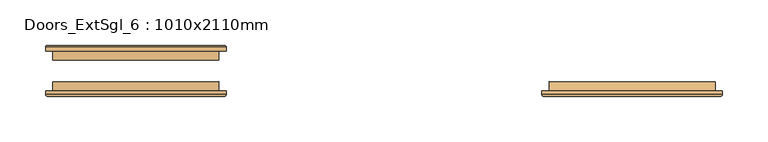
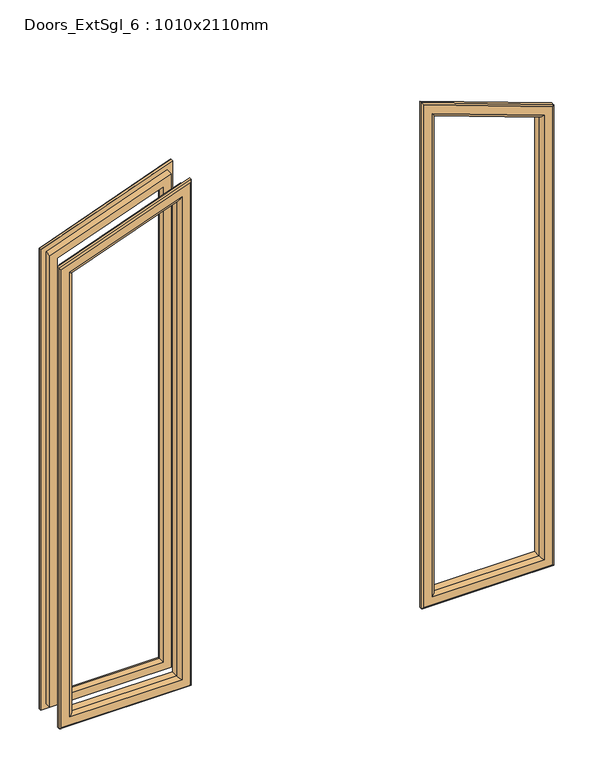
"""IFC4 building model written with IfcOpenShell, lengths in millimetres: door geometry, Doors_ExtSgl_6 : 1010x2110mm."""

from ifc_helpers import new_model, si_unit, frame, origin, place, context, project, spatial, ellipse_curve, source, transform, mapped, element, save
from ifc_brep_helpers import plane_surface, cylinder_surface, advanced_brep


def doors_extsgl_6_1010x2110mm_efbaf1af(model_context):
    return source(origin(), model_context, "Body", "AdvancedBrep", [
        advanced_brep(
        [(363.5333333, -2.4, 1776.1968198), (363.5333333, -12.4, 1776.1968198), (363.5333333, -12.4, 1058.5), (363.5333333, -2.4, 1058.5), (351.5333333, -13.4, 1767.7943294), (351.5333333, -2.4, 1767.7943294), (351.5333333, -2.4, 1070.5), (351.5333333, -13.4, 1070.5), (356.5333333, -18.4, 1771.2953671), (356.5333333, -18.4, 1065.5), (371.5333333, -16.4, 1781.7984801), (369.5333333, -18.4, 1780.3980651), (369.5333333, -18.4, 1052.5), (371.5333333, -16.4, 1050.5), (371.5333333, -12.4, 1781.7984801), (371.5333333, -12.4, 1050.5), (181.2, -12.4, 1058.5), (181.2, -2.4, 1058.5), (193.2, -2.4, 1070.5), (193.2, -13.4, 1070.5), (188.2, -18.4, 1065.5), (175.2, -18.4, 1052.5), (173.2, -16.4, 1050.5), (173.2, -12.4, 1050.5), (181.2, -12.4, 1842.5607259), (181.2, -2.4, 1842.5607259), (193.2, -2.4, 1825.4229498), (193.2, -13.4, 1825.4229498), (188.2, -18.4, 1832.5636898), (175.2, -18.4, 1851.1296139), (173.2, -16.4, 1853.9859099), (173.2, -12.4, 1853.9859099)],
        [
            (0, 1),
            (1, 2),
            (2, 3),
            (3, 0),
            (4, 5),
            (5, 6),
            (6, 7),
            (7, 4),
            (8, 4, ellipse_curve(frame((356.5333333, -13.4, 1771.2953671), z_axis=(0.5735764363510455, 0.0, -0.8191520442889922), x_axis=(0.8191520442889922, 0.0, 0.5735764363510455)), 6.1038729, 5.0)),
            (7, 9, ellipse_curve(frame((356.5333333, -13.4, 1065.5), z_axis=(0.7071067811865475, 0.0, 0.7071067811865475), x_axis=(-0.7071067811865474, 0.0, 0.7071067811865476)), 7.0710678, 5.0)),
            (9, 8),
            (10, 11, ellipse_curve(frame((369.5333333, -16.4, 1780.3980651), z_axis=(0.5735764363510455, 0.0, -0.8191520442889922), x_axis=(0.8191520442889922, 0.0, 0.5735764363510455)), 2.4415492, 2.0)),
            (11, 12),
            (12, 13, ellipse_curve(frame((369.5333333, -16.4, 1052.5), z_axis=(0.7071067811865475, 0.0, 0.7071067811865475), x_axis=(-0.7071067811865474, 0.0, 0.7071067811865476)), 2.8284271, 2.0)),
            (13, 10),
            (14, 10),
            (13, 15),
            (15, 14),
            (2, 16),
            (16, 17),
            (17, 3),
            (6, 18),
            (18, 19),
            (19, 7),
            (19, 20, ellipse_curve(frame((188.2, -13.4, 1065.5), z_axis=(0.7071067811865475, 0.0, -0.7071067811865475), x_axis=(0.7071067811865476, 0.0, 0.7071067811865474)), 7.0710678, 5.0)),
            (20, 9),
            (12, 21),
            (21, 22, ellipse_curve(frame((175.2, -16.4, 1052.5), z_axis=(0.7071067811865475, 0.0, -0.7071067811865475), x_axis=(0.7071067811865476, 0.0, 0.7071067811865474)), 2.8284271, 2.0)),
            (22, 13),
            (22, 23),
            (23, 15),
            (16, 24),
            (24, 25),
            (25, 17),
            (18, 26),
            (26, 27),
            (27, 19),
            (27, 28, ellipse_curve(frame((188.2, -13.4, 1832.5636898), z_axis=(-0.8191520442889922, 0.0, -0.5735764363510455), x_axis=(0.5735764363510455, 0.0, -0.8191520442889922)), 8.717234, 5.0)),
            (28, 20),
            (21, 29),
            (29, 30, ellipse_curve(frame((175.2, -16.4, 1851.1296139), z_axis=(-0.8191520442889922, 0.0, -0.5735764363510455), x_axis=(0.5735764363510455, 0.0, -0.8191520442889922)), 3.4868936, 2.0)),
            (30, 22),
            (30, 31),
            (31, 23),
            (31, 14),
            (1, 24),
            (0, 25),
            (5, 26),
            (4, 27),
            (8, 28),
            (11, 29),
            (10, 30),
        ],
        [
            plane_surface(frame((363.5333333, -12.4, 1776.1968198), z_axis=(1.0, 0.0, 0.0), x_axis=(0.0, 0.0, -1.0))),
            plane_surface(frame((351.5333333, -2.4, 1767.7943294), z_axis=(-1.0, 0.0, 0.0), x_axis=(0.0, 0.0, -1.0))),
            cylinder_surface(frame((356.5333333, -13.4, 1776.1968198), z_axis=(0.0, 0.0, 1.0), x_axis=(1.0, 0.0, 0.0)), 5.0),
            cylinder_surface(frame((369.5333333, -16.4, 1776.1968198), z_axis=(0.0, 0.0, 1.0), x_axis=(1.0, 0.0, 0.0)), 2.0),
            plane_surface(frame((371.5333333, -16.4, 1781.7984801), z_axis=(1.0, 0.0, 0.0), x_axis=(0.0, 0.0, -1.0))),
            plane_surface(frame((363.5333333, -12.4, 1058.5), z_axis=(0.0, 0.0, -1.0), x_axis=(-1.0, 0.0, 0.0))),
            plane_surface(frame((351.5333333, -2.4, 1070.5), z_axis=(0.0, 0.0, 1.0), x_axis=(-1.0, 0.0, 0.0))),
            cylinder_surface(frame((363.5333333, -13.4, 1065.5), z_axis=(1.0, 0.0, 0.0), x_axis=(0.0, 0.0, -1.0)), 5.0),
            cylinder_surface(frame((363.5333333, -16.4, 1052.5), z_axis=(1.0, 0.0, 0.0), x_axis=(0.0, 0.0, -1.0)), 2.0),
            plane_surface(frame((371.5333333, -16.4, 1050.5), z_axis=(0.0, 0.0, -1.0), x_axis=(-1.0, 0.0, 0.0))),
            plane_surface(frame((181.2, -12.4, 1058.5), z_axis=(-1.0, 0.0, 0.0), x_axis=(0.0, 0.0, 1.0))),
            plane_surface(frame((193.2, -2.4, 1070.5), z_axis=(1.0, 0.0, 0.0), x_axis=(0.0, 0.0, 1.0))),
            cylinder_surface(frame((188.2, -13.4, 1058.5), z_axis=(0.0, 0.0, -1.0), x_axis=(-1.0, 0.0, 0.0)), 5.0),
            cylinder_surface(frame((175.2, -16.4, 1058.5), z_axis=(0.0, 0.0, -1.0), x_axis=(-1.0, 0.0, 0.0)), 2.0),
            plane_surface(frame((173.2, -16.4, 1050.5), z_axis=(-1.0, 0.0, 0.0), x_axis=(0.0, 0.0, 1.0))),
            plane_surface(frame((173.2, -12.4, 1853.9859099), z_axis=(0.0, 1.0000000000000002, 0.0), x_axis=(0.9396926207859078, 0.0, -0.3420201433256707))),
            plane_surface(frame((181.2, -12.4, 1842.5607259), z_axis=(0.3420201433256708, 0.0, 0.9396926207859077), x_axis=(0.9396926207859077, 0.0, -0.3420201433256708))),
            plane_surface(frame((181.2, -2.4, 1842.5607259), z_axis=(0.0, 1.0000000000000002, 0.0), x_axis=(0.939692620785908, 0.0, -0.34202014332567))),
            plane_surface(frame((193.2, -2.4, 1825.4229498), z_axis=(-0.34202014332566955, 0.0, -0.9396926207859082), x_axis=(0.9396926207859082, 0.0, -0.34202014332566955))),
            cylinder_surface(frame((178.805859, -13.4, 1835.9828775), z_axis=(-0.9396926207859079, 0.0, 0.34202014332567016), x_axis=(0.34202014332567016, 0.0, 0.9396926207859079)), 5.0),
            plane_surface(frame((188.2, -18.4, 1832.5636898), z_axis=(0.0, -1.0, 0.0), x_axis=(0.9396926207859079, 0.0, -0.34202014332567027))),
            cylinder_surface(frame((183.2521209, -16.4, 1848.1988816), z_axis=(-0.9396926207859079, 0.0, 0.34202014332567016), x_axis=(0.34202014332567016, 0.0, 0.9396926207859079)), 2.0),
            plane_surface(frame((173.2, -16.4, 1853.9859099), z_axis=(0.3420201433256701, 0.0, 0.939692620785908), x_axis=(0.939692620785908, 0.0, -0.3420201433256701))),
        ],
        [
            (0, [[1, 2, 3, 4]]),
            (1, [[5, 6, 7, 8]]),
            (2, [[9, -8, 10, 11]]),
            (3, [[12, 13, 14, 15]]),
            (4, [[16, -15, 17, 18]]),
            (5, [[-3, 19, 20, 21]]),
            (6, [[-7, 22, 23, 24]]),
            (7, [[-10, -24, 25, 26]]),
            (8, [[-14, 27, 28, 29]]),
            (9, [[-17, -29, 30, 31]]),
            (10, [[-20, 32, 33, 34]]),
            (11, [[-23, 35, 36, 37]]),
            (12, [[-25, -37, 38, 39]]),
            (13, [[-28, 40, 41, 42]]),
            (14, [[-30, -42, 43, 44]]),
            (15, [[-31, -44, 45, -18], [46, -32, -19, -2]]),
            (16, [[-33, -46, -1, 47]]),
            (17, [[-21, -34, -47, -4], [48, -35, -22, -6]]),
            (18, [[-36, -48, -5, 49]]),
            (19, [[-38, -49, -9, 50]]),
            (20, [[51, -40, -27, -13], [-26, -39, -50, -11]]),
            (21, [[-41, -51, -12, 52]]),
            (22, [[-43, -52, -16, -45]]),
        ],
    ),
        advanced_brep(
        [(-173.1333333, 35.6, 1050.5), (-173.1333333, 31.6, 1050.5), (-371.4666667, 31.6, 1050.5), (-371.4666667, 35.6, 1050.5), (-175.1333333, 37.6, 1052.5), (-369.4666667, 37.6, 1052.5), (-193.1333333, 32.6, 1070.5), (-188.1333333, 37.6, 1065.5), (-356.4666667, 37.6, 1065.5), (-351.4666667, 32.6, 1070.5), (-193.1333333, 21.6, 1070.5), (-351.4666667, 21.6, 1070.5), (-181.1333333, 31.6, 1058.5), (-181.1333333, 21.6, 1058.5), (-363.4666667, 21.6, 1058.5), (-363.4666667, 31.6, 1058.5), (-371.4666667, 31.6, 1781.7984801), (-371.4666667, 35.6, 1781.7984801), (-369.4666667, 37.6, 1780.3980651), (-356.4666667, 37.6, 1771.2953671), (-351.4666667, 32.6, 1767.7943294), (-351.4666667, 21.6, 1767.7943294), (-363.4666667, 21.6, 1776.1968198), (-363.4666667, 31.6, 1776.1968198), (-173.1333333, 31.6, 1853.9859099), (-173.1333333, 35.6, 1853.9859099), (-175.1333333, 37.6, 1851.1296139), (-188.1333333, 37.6, 1832.5636898), (-193.1333333, 32.6, 1825.4229498), (-193.1333333, 21.6, 1825.4229498), (-181.1333333, 21.6, 1842.5607259), (-181.1333333, 31.6, 1842.5607259)],
        [
            (0, 1),
            (1, 2),
            (2, 3),
            (3, 0),
            (4, 0, ellipse_curve(frame((-175.1333333, 35.6, 1052.5), z_axis=(-0.7071067811865475, 0.0, -0.7071067811865475), x_axis=(0.7071067811865477, 0.0, -0.7071067811865474)), 2.8284271, 2.0)),
            (3, 5, ellipse_curve(frame((-369.4666667, 35.6, 1052.5), z_axis=(0.7071067811865475, 0.0, -0.7071067811865475), x_axis=(0.7071067811865476, 0.0, 0.7071067811865474)), 2.8284271, 2.0)),
            (5, 4),
            (6, 7, ellipse_curve(frame((-188.1333333, 32.6, 1065.5), z_axis=(-0.7071067811865475, 0.0, -0.7071067811865475), x_axis=(0.7071067811865477, 0.0, -0.7071067811865474)), 7.0710678, 5.0)),
            (7, 8),
            (8, 9, ellipse_curve(frame((-356.4666667, 32.6, 1065.5), z_axis=(0.7071067811865475, 0.0, -0.7071067811865475), x_axis=(0.7071067811865476, 0.0, 0.7071067811865474)), 7.0710678, 5.0)),
            (9, 6),
            (10, 6),
            (9, 11),
            (11, 10),
            (12, 13),
            (13, 14),
            (14, 15),
            (15, 12),
            (2, 16),
            (16, 17),
            (17, 3),
            (17, 18, ellipse_curve(frame((-369.4666667, 35.6, 1780.3980651), z_axis=(-0.5735764363510453, 0.0, -0.8191520442889925), x_axis=(0.8191520442889926, 0.0, -0.573576436351045)), 2.4415492, 2.0)),
            (18, 5),
            (8, 19),
            (19, 20, ellipse_curve(frame((-356.4666667, 32.6, 1771.2953671), z_axis=(-0.5735764363510453, 0.0, -0.8191520442889925), x_axis=(0.8191520442889926, 0.0, -0.573576436351045)), 6.1038729, 5.0)),
            (20, 9),
            (20, 21),
            (21, 11),
            (14, 22),
            (22, 23),
            (23, 15),
            (16, 24),
            (24, 25),
            (25, 17),
            (25, 26, ellipse_curve(frame((-175.1333333, 35.6, 1851.1296139), z_axis=(-0.8191520442889926, 0.0, 0.5735764363510452), x_axis=(-0.5735764363510449, 0.0, -0.8191520442889927)), 3.4868936, 2.0)),
            (26, 18),
            (19, 27),
            (27, 28, ellipse_curve(frame((-188.1333333, 32.6, 1832.5636898), z_axis=(-0.8191520442889926, 0.0, 0.5735764363510452), x_axis=(-0.5735764363510449, 0.0, -0.8191520442889927)), 8.717234, 5.0)),
            (28, 20),
            (28, 29),
            (29, 21),
            (22, 30),
            (30, 31),
            (31, 23),
            (24, 1),
            (0, 25),
            (4, 26),
            (7, 27),
            (6, 28),
            (10, 29),
            (13, 30),
            (12, 31),
        ],
        [
            plane_surface(frame((-173.1333333, 31.6, 1050.5), z_axis=(0.0, 0.0, -1.0), x_axis=(-1.0, 0.0, 0.0))),
            cylinder_surface(frame((-181.1333333, 35.6, 1052.5), z_axis=(1.0, 0.0, 0.0), x_axis=(0.0, 0.0, -1.0)), 2.0),
            cylinder_surface(frame((-181.1333333, 32.6, 1065.5), z_axis=(1.0, 0.0, 0.0), x_axis=(0.0, 0.0, -1.0)), 5.0),
            plane_surface(frame((-193.1333333, 32.6, 1070.5), z_axis=(0.0, 0.0, 1.0), x_axis=(-1.0, 0.0, 0.0))),
            plane_surface(frame((-181.1333333, 21.6, 1058.5), z_axis=(0.0, 0.0, -1.0), x_axis=(-1.0, 0.0, 0.0))),
            plane_surface(frame((-371.4666667, 31.6, 1050.5), z_axis=(-1.0, 0.0, 0.0), x_axis=(0.0, 0.0, 1.0))),
            cylinder_surface(frame((-369.4666667, 35.6, 1058.5), z_axis=(0.0, 0.0, -1.0), x_axis=(-1.0, 0.0, 0.0)), 2.0),
            cylinder_surface(frame((-356.4666667, 32.6, 1058.5), z_axis=(0.0, 0.0, -1.0), x_axis=(-1.0, 0.0, 0.0)), 5.0),
            plane_surface(frame((-351.4666667, 32.6, 1070.5), z_axis=(1.0, 0.0, 0.0), x_axis=(0.0, 0.0, 1.0))),
            plane_surface(frame((-363.4666667, 21.6, 1058.5), z_axis=(-1.0, 0.0, 0.0), x_axis=(0.0, 0.0, 1.0))),
            plane_surface(frame((-371.4666667, 31.6, 1781.7984801), z_axis=(-0.3420201433256706, 0.0, 0.9396926207859078), x_axis=(0.9396926207859078, 0.0, 0.3420201433256706))),
            cylinder_surface(frame((-365.5187875, 35.6, 1781.8349756), z_axis=(-0.9396926207859077, 0.0, -0.3420201433256709), x_axis=(-0.3420201433256709, 0.0, 0.9396926207859077)), 2.0),
            cylinder_surface(frame((-361.0725257, 32.6, 1769.6189715), z_axis=(-0.9396926207859077, 0.0, -0.3420201433256709), x_axis=(-0.3420201433256709, 0.0, 0.9396926207859077)), 5.0),
            plane_surface(frame((-351.4666667, 32.6, 1767.7943294), z_axis=(0.34202014332567116, 0.0, -0.9396926207859075), x_axis=(0.9396926207859075, 0.0, 0.34202014332567116))),
            plane_surface(frame((-363.4666667, 21.6, 1776.1968198), z_axis=(-0.3420201433256707, 0.0, 0.9396926207859078), x_axis=(0.9396926207859078, 0.0, 0.3420201433256707))),
            plane_surface(frame((-173.1333333, 31.6, 1853.9859099), z_axis=(1.0, 0.0, 0.0), x_axis=(0.0, 0.0, -1.0))),
            cylinder_surface(frame((-175.1333333, 35.6, 1842.5607259), z_axis=(0.0, 0.0, 1.0), x_axis=(1.0, 0.0, 0.0)), 2.0),
            plane_surface(frame((-175.1333333, 37.6, 1851.1296139), z_axis=(0.0, 1.0, 0.0), x_axis=(0.0, 0.0, -1.0))),
            cylinder_surface(frame((-188.1333333, 32.6, 1842.5607259), z_axis=(0.0, 0.0, 1.0), x_axis=(1.0, 0.0, 0.0)), 5.0),
            plane_surface(frame((-193.1333333, 32.6, 1825.4229498), z_axis=(-1.0, 0.0, 0.0), x_axis=(0.0, 0.0, -1.0))),
            plane_surface(frame((-193.1333333, 21.6, 1825.4229498), z_axis=(0.0, -1.0, 0.0), x_axis=(0.0, 0.0, -1.0))),
            plane_surface(frame((-181.1333333, 21.6, 1842.5607259), z_axis=(1.0, 0.0, 0.0), x_axis=(0.0, 0.0, -1.0))),
            plane_surface(frame((-181.1333333, 31.6, 1842.5607259), z_axis=(0.0, -1.0, 0.0), x_axis=(0.0, 0.0, -1.0))),
        ],
        [
            (0, [[1, 2, 3, 4]]),
            (1, [[5, -4, 6, 7]]),
            (2, [[8, 9, 10, 11]]),
            (3, [[12, -11, 13, 14]]),
            (4, [[15, 16, 17, 18]]),
            (5, [[-3, 19, 20, 21]]),
            (6, [[-6, -21, 22, 23]]),
            (7, [[-10, 24, 25, 26]]),
            (8, [[-13, -26, 27, 28]]),
            (9, [[-17, 29, 30, 31]]),
            (10, [[-20, 32, 33, 34]]),
            (11, [[-22, -34, 35, 36]]),
            (12, [[-25, 37, 38, 39]]),
            (13, [[-27, -39, 40, 41]]),
            (14, [[-30, 42, 43, 44]]),
            (15, [[-33, 45, -1, 46]]),
            (16, [[-35, -46, -5, 47]]),
            (17, [[-23, -36, -47, -7], [48, -37, -24, -9]]),
            (18, [[-38, -48, -8, 49]]),
            (19, [[-40, -49, -12, 50]]),
            (20, [[51, -42, -29, -16], [-28, -41, -50, -14]]),
            (21, [[-43, -51, -15, 52]]),
            (22, [[-45, -32, -19, -2], [-31, -44, -52, -18]]),
        ],
    ),
        advanced_brep(
        [(-363.4666667, -2.4, 1776.1968198), (-363.4666667, -12.4, 1776.1968198), (-181.1333333, -12.4, 1842.5607259), (-181.1333333, -2.4, 1842.5607259), (-351.4666667, -13.4, 1767.7943294), (-351.4666667, -2.4, 1767.7943294), (-193.1333333, -2.4, 1825.4229498), (-193.1333333, -13.4, 1825.4229498), (-356.4666667, -18.4, 1771.2953671), (-188.1333333, -18.4, 1832.5636898), (-371.4666667, -16.4, 1781.7984801), (-369.4666667, -18.4, 1780.3980651), (-175.1333333, -18.4, 1851.1296139), (-173.1333333, -16.4, 1853.9859099), (-371.4666667, -12.4, 1781.7984801), (-173.1333333, -12.4, 1853.9859099), (-181.1333333, -12.4, 1058.5), (-181.1333333, -2.4, 1058.5), (-193.1333333, -2.4, 1070.5), (-193.1333333, -13.4, 1070.5), (-188.1333333, -18.4, 1065.5), (-175.1333333, -18.4, 1052.5), (-173.1333333, -16.4, 1050.5), (-173.1333333, -12.4, 1050.5), (-363.4666667, -12.4, 1058.5), (-363.4666667, -2.4, 1058.5), (-351.4666667, -2.4, 1070.5), (-351.4666667, -13.4, 1070.5), (-356.4666667, -18.4, 1065.5), (-369.4666667, -18.4, 1052.5), (-371.4666667, -16.4, 1050.5), (-371.4666667, -12.4, 1050.5)],
        [
            (0, 1),
            (1, 2),
            (2, 3),
            (3, 0),
            (4, 5),
            (5, 6),
            (6, 7),
            (7, 4),
            (8, 4, ellipse_curve(frame((-356.4666667, -13.4, 1771.2953671), z_axis=(0.5735764363510453, 0.0, 0.8191520442889927), x_axis=(-0.819152044288992, 0.0, 0.5735764363510456)), 6.1038729, 5.0)),
            (7, 9, ellipse_curve(frame((-188.1333333, -13.4, 1832.5636898), z_axis=(-0.8191520442889926, 0.0, 0.5735764363510449), x_axis=(-0.5735764363510449, 0.0, -0.8191520442889927)), 8.717234, 5.0)),
            (9, 8),
            (10, 11, ellipse_curve(frame((-369.4666667, -16.4, 1780.3980651), z_axis=(0.5735764363510453, 0.0, 0.8191520442889927), x_axis=(-0.819152044288992, 0.0, 0.5735764363510456)), 2.4415492, 2.0)),
            (11, 12),
            (12, 13, ellipse_curve(frame((-175.1333333, -16.4, 1851.1296139), z_axis=(-0.8191520442889926, 0.0, 0.5735764363510449), x_axis=(-0.5735764363510449, 0.0, -0.8191520442889927)), 3.4868936, 2.0)),
            (13, 10),
            (14, 10),
            (13, 15),
            (15, 14),
            (2, 16),
            (16, 17),
            (17, 3),
            (6, 18),
            (18, 19),
            (19, 7),
            (19, 20, ellipse_curve(frame((-188.1333333, -13.4, 1065.5), z_axis=(0.7071067811865475, 0.0, 0.7071067811865475), x_axis=(-0.7071067811865474, 0.0, 0.7071067811865476)), 7.0710678, 5.0)),
            (20, 9),
            (12, 21),
            (21, 22, ellipse_curve(frame((-175.1333333, -16.4, 1052.5), z_axis=(0.7071067811865475, 0.0, 0.7071067811865475), x_axis=(-0.7071067811865474, 0.0, 0.7071067811865476)), 2.8284271, 2.0)),
            (22, 13),
            (22, 23),
            (23, 15),
            (16, 24),
            (24, 25),
            (25, 17),
            (18, 26),
            (26, 27),
            (27, 19),
            (27, 28, ellipse_curve(frame((-356.4666667, -13.4, 1065.5), z_axis=(0.7071067811865475, 0.0, -0.7071067811865475), x_axis=(0.7071067811865476, 0.0, 0.7071067811865474)), 7.0710678, 5.0)),
            (28, 20),
            (21, 29),
            (29, 30, ellipse_curve(frame((-369.4666667, -16.4, 1052.5), z_axis=(0.7071067811865475, 0.0, -0.7071067811865475), x_axis=(0.7071067811865476, 0.0, 0.7071067811865474)), 2.8284271, 2.0)),
            (30, 22),
            (30, 31),
            (31, 23),
            (31, 14),
            (1, 24),
            (0, 25),
            (5, 26),
            (4, 27),
            (8, 28),
            (11, 29),
            (10, 30),
        ],
        [
            plane_surface(frame((-363.4666667, -12.4, 1776.1968198), z_axis=(-0.34202014332566993, 0.0, 0.939692620785908), x_axis=(0.939692620785908, 0.0, 0.34202014332566993))),
            plane_surface(frame((-351.4666667, -2.4, 1767.7943294), z_axis=(0.3420201433256702, 0.0, -0.9396926207859079), x_axis=(0.9396926207859079, 0.0, 0.3420201433256702))),
            cylinder_surface(frame((-361.0725257, -13.4, 1769.6189715), z_axis=(-0.9396926207859077, 0.0, -0.34202014332567104), x_axis=(-0.34202014332567104, 0.0, 0.9396926207859077)), 5.0),
            cylinder_surface(frame((-365.5187875, -16.4, 1781.8349756), z_axis=(-0.9396926207859077, 0.0, -0.34202014332567104), x_axis=(-0.34202014332567104, 0.0, 0.9396926207859077)), 2.0),
            plane_surface(frame((-371.4666667, -16.4, 1781.7984801), z_axis=(-0.34202014332567143, 0.0, 0.9396926207859074), x_axis=(0.9396926207859074, 0.0, 0.34202014332567143))),
            plane_surface(frame((-181.1333333, -12.4, 1842.5607259), z_axis=(1.0, 0.0, 0.0), x_axis=(0.0, 0.0, -1.0))),
            plane_surface(frame((-193.1333333, -2.4, 1825.4229498), z_axis=(-1.0, 0.0, 0.0), x_axis=(0.0, 0.0, -1.0))),
            cylinder_surface(frame((-188.1333333, -13.4, 1842.5607259), z_axis=(0.0, 0.0, 1.0), x_axis=(1.0, 0.0, 0.0)), 5.0),
            cylinder_surface(frame((-175.1333333, -16.4, 1842.5607259), z_axis=(0.0, 0.0, 1.0), x_axis=(1.0, 0.0, 0.0)), 2.0),
            plane_surface(frame((-173.1333333, -16.4, 1853.9859099), z_axis=(1.0, 0.0, 0.0), x_axis=(0.0, 0.0, -1.0))),
            plane_surface(frame((-181.1333333, -12.4, 1058.5), z_axis=(0.0, 0.0, -1.0), x_axis=(-1.0, 0.0, 0.0))),
            plane_surface(frame((-193.1333333, -2.4, 1070.5), z_axis=(0.0, 0.0, 1.0), x_axis=(-1.0, 0.0, 0.0))),
            cylinder_surface(frame((-181.1333333, -13.4, 1065.5), z_axis=(1.0, 0.0, 0.0), x_axis=(0.0, 0.0, -1.0)), 5.0),
            cylinder_surface(frame((-181.1333333, -16.4, 1052.5), z_axis=(1.0, 0.0, 0.0), x_axis=(0.0, 0.0, -1.0)), 2.0),
            plane_surface(frame((-173.1333333, -16.4, 1050.5), z_axis=(0.0, 0.0, -1.0), x_axis=(-1.0, 0.0, 0.0))),
            plane_surface(frame((-371.4666667, -12.4, 1050.5), z_axis=(0.0, 1.0, 0.0), x_axis=(0.0, 0.0, 1.0))),
            plane_surface(frame((-363.4666667, -12.4, 1058.5), z_axis=(-1.0, 0.0, 0.0), x_axis=(0.0, 0.0, 1.0))),
            plane_surface(frame((-363.4666667, -2.4, 1058.5), z_axis=(0.0, 1.0, 0.0), x_axis=(0.0, 0.0, 1.0))),
            plane_surface(frame((-351.4666667, -2.4, 1070.5), z_axis=(1.0, 0.0, 0.0), x_axis=(0.0, 0.0, 1.0))),
            cylinder_surface(frame((-356.4666667, -13.4, 1058.5), z_axis=(0.0, 0.0, -1.0), x_axis=(-1.0, 0.0, 0.0)), 5.0),
            plane_surface(frame((-356.4666667, -18.4, 1065.5), z_axis=(0.0, -1.0, 0.0), x_axis=(0.0, 0.0, 1.0))),
            cylinder_surface(frame((-369.4666667, -16.4, 1058.5), z_axis=(0.0, 0.0, -1.0), x_axis=(-1.0, 0.0, 0.0)), 2.0),
            plane_surface(frame((-371.4666667, -16.4, 1050.5), z_axis=(-1.0, 0.0, 0.0), x_axis=(0.0, 0.0, 1.0))),
        ],
        [
            (0, [[1, 2, 3, 4]]),
            (1, [[5, 6, 7, 8]]),
            (2, [[9, -8, 10, 11]]),
            (3, [[12, 13, 14, 15]]),
            (4, [[16, -15, 17, 18]]),
            (5, [[-3, 19, 20, 21]]),
            (6, [[-7, 22, 23, 24]]),
            (7, [[-10, -24, 25, 26]]),
            (8, [[-14, 27, 28, 29]]),
            (9, [[-17, -29, 30, 31]]),
            (10, [[-20, 32, 33, 34]]),
            (11, [[-23, 35, 36, 37]]),
            (12, [[-25, -37, 38, 39]]),
            (13, [[-28, 40, 41, 42]]),
            (14, [[-30, -42, 43, 44]]),
            (15, [[-31, -44, 45, -18], [46, -32, -19, -2]]),
            (16, [[-33, -46, -1, 47]]),
            (17, [[-21, -34, -47, -4], [48, -35, -22, -6]]),
            (18, [[-36, -48, -5, 49]]),
            (19, [[-38, -49, -9, 50]]),
            (20, [[51, -40, -27, -13], [-26, -39, -50, -11]]),
            (21, [[-41, -51, -12, 52]]),
            (22, [[-43, -52, -16, -45]]),
        ],
    ),
    ])


if __name__ == "__main__":
    model = new_model("IFC4")
    model_context = context("Model", 3, world=origin())
    ifc_project = project(units=[si_unit("LENGTHUNIT", "METRE", prefix="MILLI")], contexts=[model_context])
    site = spatial("IfcSite", under=ifc_project)
    building = spatial("IfcBuilding", under=site)
    placement = place(None, origin())
    doors_extsgl_6_1010x2110mm_shape = doors_extsgl_6_1010x2110mm_efbaf1af(model_context)
    element("IfcDoor", 1, ObjectType="Doors_ExtSgl_6 : 1010x2110mm", at=placement, inside=building, context=model_context, shape_type="MappedRepresentation", body=[
        mapped(doors_extsgl_6_1010x2110mm_shape, transform((0.0, 0.0, 0.0), x_axis=(1.0, 0.0, 0.0), y_axis=(0.0, 1.0, 0.0), z_axis=(0.0, 0.0, 1.0))),
    ])
    save(model, "model.ifc")

# Revit data of these elements
# Type "Doors_ExtSgl_6 : 1010x2110mm"
#   Type Mark = "12"
#   Type Comments = "External Single"
#   Operation = "SingleSwingRight"
#   Construction Type Id = "SGL"
#   Keynote = "L20"
#   Analytic Construction = "Large single-glazed windows"
#   Wrap Layers (Int) from Ext = 0' - 6.98819"
#   Wrap Layers (Ext) from Ext = 0' - 4.03543"
#   Visual Light Transmittance = 0.9
#   Thickness = 0' - 1.73228"
#   Stile Top of Lock rail = 3' - 3.37008"
#   Stile Top Rail = 0' - 5.90551"
#   Stile Shutting = 0' - 3.54331"
#   Stile Muntin Rail = 0' - 3.54331"
#   Stile Lock Rail = 0' - 6.88976"
#   Stile Hanging = 0' - 3.54331"
#   Stile Bottom Rail = 0' - 6.88976"
#   Solar Heat Gain Coefficient = 0.86
#   Rough Width = 3' - 3.76378"
#   Rough Height = 6' - 11.07087"
#   O/A Frame Width = 0' - 2.51969"
#   Heat Transfer Coefficient (U) = 0.979472 BTU/(h·ft²·°F)
#   Handle Z Distance = 3' - 3.37008"
#   Glazing Thickness = 0' - 0.94488"
#   FrameWidth = 0' - 1.65354"
#   FrameOffset - External = 0' - 0.98425"
#   FrameDepth = 0' - 3.50394"
#   Door Panel Width = 2' - 11.70866"
#   Door Panel Thickness = 0' - 1.73228"
#   Door Panel Height = 6' - 6.74016"
#   DONT CHANGE - Panel Width = 0' - 7.17848"
#   Cill Thickness = 0' - 2.14567"
#   Cill Projection = 0' - 1.1811"
#   Handle X Distance = 0' - 2.95276"
#   Height = 6' - 11.07087"
#   Structural Tolerance = 0' - 0.25591"
#   Tolerance = 0' - 0.11811"
#   Undercut = 0' - 0.15748"
#   Width = 3' - 3.76378"
#   Cill Extension = 0' - 0.98425"
#   Cavity Closer Width = 0' - 1.9685"
#   Cavity Closer Offset from Ext = 0' - 4.03543"
#   Cavity Closer Depth = 0' - 3.34646"
#   Vis - Ironmongery = yes
#   Vis - Cavity Closers = yes
#   Define Thermal Properties by = 1
#   Function = 1
#   Material Glass = Door - Glazing
#   Material Door = Door - Panel
#   Material Frame = Door - Frame/Mullion
#   Material Ironmongery = Door - Handle
#   Wall Closure = (empty or 0)
# Element 1 (IfcDoor, "Doors_ExtSgl_6 : 1010x2110mm")
#   Materials on its faces: "Door - Panel", "Door - Handle", "Door - Frame/Mullion", "Door - Glazing"
# Materials
#   "Door - Glazing": colour RGB 0 0 255, transparency 0.75
#   "Door - Panel": class "Wood", colour RGB 210 159 95, transparency 0, Cost = 0
#   "Door - Frame/Mullion": class "Wood", colour RGB 212 179 113, transparency 0
#   "Door - Handle": colour RGB 0 0 0, transparency 0
